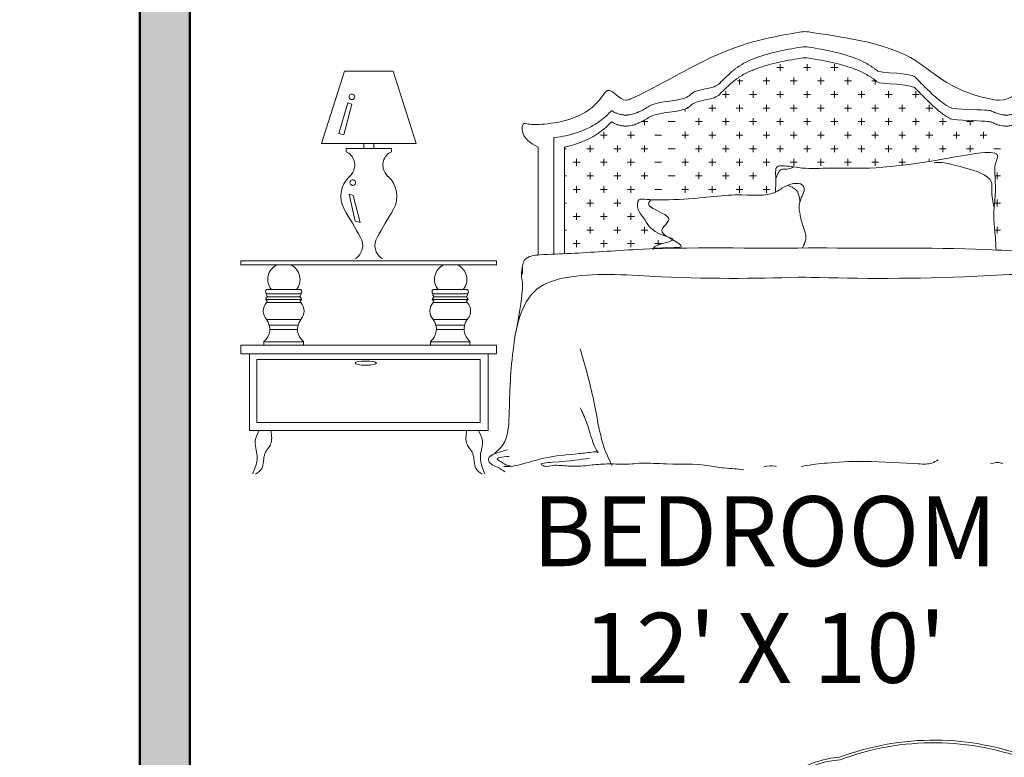
# Model space of a CAD drawing. Units: inches. Extents: x 1771 to 3025, y 319 to 889.
# Tile 33 of 35: x 2854 to 2952, y 714 to 788. Entities that reach past the tile are written whole.
import ezdxf

# ---------------------------------------------------------------- set-up
doc = ezdxf.new("R2010")
doc.units = ezdxf.units.IN
doc.header["$MEASUREMENT"] = 0
doc.set_wipeout_variables(frame=1)
for name, color, linetype, lineweight in [('A-AREA-IDEN', 241, 'Continuous', 25), ('A-FURN', 8, 'Continuous', 18), ('A-WALL', 7, 'Continuous', 50), ('A-WALL-PATT', 254, 'Continuous', 13)]:
    doc.layers.add(name, color=color, linetype=linetype, lineweight=lineweight)
doc.styles.get("Standard").update_dxf_attribs({"font": 'arial.ttf'})

# ---------------------------------------------------------------- blocks, each defined once
blk = doc.blocks.new('A$C3F6F0378')
for p, q in [((1198.7, 944.7), (1198.7, 946.2)), ((1254.2, 952.6), (1270.1, 952.6)), ((1262.2, 944.7), (1262.2, 960.5)), ((1317.7, 952.6), (1333.6, 952.6)), ((1325.7, 944.7), (1325.7, 960.5)), ((1381.2, 952.6), (1397.1, 952.6)), ((1389.2, 944.7), (1389.2, 959.9)), ((188.6, 774.2), (242.7, 943.6)), ((356.2, 943.6), (242.7, 943.6)), ((410.4, 774.2), (356.2, 943.6)), ((1166.9, 912.9), (1166.9, 924)), ((1230.4, 912.9), (1230.4, 928.8)), ((1293.9, 912.9), (1293.9, 928.8)), ((1357.4, 912.9), (1357.4, 928.8)), ((1420.9, 912.9), (1420.9, 928.8)), ((1162.7, 920.9), (1174.9, 920.9)), ((1222.5, 920.9), (1238.4, 920.9)), ((1286, 920.9), (1301.9, 920.9)), ((1349.5, 920.9), (1365.4, 920.9)), ((1413, 920.9), (1428.9, 920.9)), ((1476.5, 920.9), (1485.8, 920.9)), ((1484.4, 912.9), (1484.4, 921.6)), ((1127.2, 889.1), (1143.1, 889.1)), ((1135.2, 881.2), (1135.2, 897)), ((1190.7, 889.1), (1206.6, 889.1)), ((1198.7, 881.2), (1198.7, 897)), ((1254.2, 889.1), (1270.1, 889.1)), ((1262.2, 881.2), (1262.2, 897)), ((1317.7, 889.1), (1333.6, 889.1)), ((1325.7, 881.2), (1325.7, 897)), ((1381.2, 889.1), (1397.1, 889.1)), ((1389.2, 881.2), (1389.2, 897)), ((1444.7, 889.1), (1460.6, 889.1)), ((1452.7, 881.2), (1452.7, 897)), ((1508.2, 889.1), (1524.1, 889.1)), ((1516.2, 881.2), (1516.2, 897)), ((1571.7, 889.1), (1587.6, 889.1)), ((1579.7, 881.2), (1579.7, 897)), ((229, 797.8), (250.3, 869.3)), ((259.4, 866.2), (241.2, 794.8)), ((250.3, 869.3), (259.4, 866.2)), ((1039.9, 849.4), (1039.9, 855.2)), ((1044.6, 857.4), (1047.9, 857.4)), ((1095.5, 857.4), (1111.4, 857.4)), ((1103.4, 849.4), (1103.4, 865.3)), ((1159, 857.4), (1174.9, 857.4)), ((1166.9, 849.4), (1166.9, 865.3)), ((1222.5, 857.4), (1238.4, 857.4)), ((1230.4, 849.4), (1230.4, 865.3)), ((1286, 857.4), (1301.9, 857.4)), ((1293.9, 849.4), (1293.9, 865.3)), ((1349.5, 857.4), (1365.4, 857.4)), ((1357.4, 849.4), (1357.4, 865.3)), ((1413, 857.4), (1428.9, 857.4)), ((1420.9, 849.4), (1420.9, 865.3)), ((1476.5, 857.4), (1492.4, 857.4)), ((1484.4, 849.4), (1484.4, 865.3)), ((1540, 857.4), (1555.9, 857.4)), ((1547.9, 849.4), (1547.9, 865.3)), ((1603.5, 857.4), (1619.4, 857.4)), ((1611.4, 849.4), (1611.4, 865.3)), ((1071.7, 817.7), (1071.7, 833.5)), ((1135.2, 817.7), (1135.2, 833.5)), ((1198.7, 817.7), (1198.7, 833.5)), ((1262.2, 817.7), (1262.2, 833.5)), ((1325.7, 817.7), (1325.7, 833.5)), ((1389.2, 817.7), (1389.2, 833.5)), ((1452.7, 817.7), (1452.7, 833.5)), ((1516.2, 817.7), (1516.2, 833.5)), ((1579.7, 817.7), (1579.7, 833.5)), ((1643.2, 817.7), (1643.2, 833.5)), ((881.2, 817.7), (881.2, 818.8)), ((937.5, 825.6), (952.6, 825.6)), ((944.7, 817.7), (944.7, 829.4)), ((1000.2, 825.6), (1016.1, 825.6)), ((1063.7, 825.6), (1079.6, 825.6)), ((1127.2, 825.6), (1143.1, 825.6)), ((1190.7, 825.6), (1206.6, 825.6)), ((1254.2, 825.6), (1270.1, 825.6)), ((1317.7, 825.6), (1333.6, 825.6)), ((1381.2, 825.6), (1397.1, 825.6)), ((1444.7, 825.6), (1460.6, 825.6)), ((1508.2, 825.6), (1524.1, 825.6)), ((1571.7, 825.6), (1587.6, 825.6)), ((1635.2, 825.6), (1651.1, 825.6)), ((1698.7, 825.6), (1714.6, 825.6)), ((1706.7, 817.7), (1706.7, 828.2)), ((1770.2, 818.9), (1770.2, 818.9)), ((241.2, 794.8), (229, 797.8)), ((841.5, 793.9), (857.4, 793.9)), ((849.4, 785.9), (849.4, 801.8)), ((905, 793.9), (920.9, 793.9)), ((912.9, 785.9), (912.9, 801.8)), ((968.5, 793.9), (984.4, 793.9)), ((1032, 793.9), (1047.9, 793.9)), ((1039.9, 785.9), (1039.9, 801.8)), ((1095.5, 793.9), (1111.4, 793.9)), ((1103.4, 785.9), (1103.4, 801.8)), ((1159, 793.9), (1174.9, 793.9)), ((1166.9, 785.9), (1166.9, 801.8)), ((1222.5, 793.9), (1238.4, 793.9)), ((1230.4, 785.9), (1230.4, 801.8)), ((1286, 793.9), (1301.9, 793.9)), ((1293.9, 785.9), (1293.9, 801.8)), ((1349.5, 793.9), (1365.4, 793.9)), ((1357.4, 785.9), (1357.4, 801.8)), ((1413, 793.9), (1428.9, 793.9)), ((1420.9, 785.9), (1420.9, 801.8)), ((1476.5, 793.9), (1492.4, 793.9)), ((1484.4, 785.9), (1484.4, 801.8)), ((1540, 793.9), (1555.9, 793.9)), ((1547.9, 785.9), (1547.9, 801.8)), ((1603.5, 793.9), (1619.4, 793.9)), ((1611.4, 785.9), (1611.4, 801.8)), ((1667, 793.9), (1682.9, 793.9)), ((1674.9, 785.9), (1674.9, 801.8)), ((1730.5, 793.9), (1746.4, 793.9)), ((1738.4, 785.9), (1738.4, 801.8)), ((410.4, 774.2), (188.6, 774.2)), ((246.2, 763), (246.2, 755.2)), ((246.2, 763), (246.2, 755.2)), ((352.5, 763), (246.2, 763)), ((287.7, 774.2), (287.7, 763)), ((311, 763), (287.7, 763)), ((311, 774.2), (311, 763)), ((352.5, 763), (352.5, 755.2)), ((352.5, 763), (352.5, 755.2)), ((757.1, 762.1), (762.1, 762.1)), ((809.7, 762.1), (825.6, 762.1)), ((817.7, 754.2), (817.7, 770)), ((873.2, 762.1), (889.1, 762.1)), ((881.2, 754.2), (881.2, 770)), ((936.7, 762.1), (952.6, 762.1)), ((944.7, 754.2), (944.7, 770)), ((1000.2, 762.1), (1016.1, 762.1)), ((1063.7, 762.1), (1079.6, 762.1)), ((1071.7, 754.2), (1071.7, 770)), ((1127.2, 762.1), (1143.1, 762.1)), ((1135.2, 754.2), (1135.2, 770)), ((1190.7, 762.1), (1206.6, 762.1)), ((1198.7, 754.2), (1198.7, 770)), ((1254.2, 762.1), (1270.1, 762.1)), ((1262.2, 754.2), (1262.2, 770)), ((1317.7, 762.1), (1333.6, 762.1)), ((1325.7, 754.2), (1325.7, 770)), ((1381.2, 762.1), (1397.1, 762.1)), ((1389.2, 754.2), (1389.2, 770)), ((1444.7, 762.1), (1460.6, 762.1)), ((1452.7, 754.2), (1452.7, 770)), ((1508.2, 762.1), (1524.1, 762.1)), ((1516.2, 754.2), (1516.2, 770)), ((1571.7, 762.1), (1587.6, 762.1)), ((1579.7, 754.2), (1579.7, 770)), ((1635.2, 762.1), (1651.1, 762.1)), ((1643.2, 754.2), (1643.2, 770)), ((1698.7, 762.1), (1714.6, 762.1)), ((1706.7, 754.2), (1706.7, 770)), ((1762.2, 762.1), (1778.1, 762.1)), ((785.9, 722.4), (785.9, 738.3)), ((849.4, 722.4), (849.4, 738.3)), ((912.9, 722.4), (912.9, 738.3)), ((1039.9, 722.4), (1039.9, 738.3)), ((1103.4, 722.4), (1103.4, 738.3)), ((1166.9, 722.4), (1166.9, 738.3)), ((1230.4, 722.4), (1230.4, 738.3)), ((1293.9, 722.4), (1293.9, 738.3)), ((1357.4, 722.4), (1357.4, 738.3)), ((1420.9, 722.4), (1420.9, 738.3)), ((1484.4, 722.4), (1484.4, 738.3)), ((1547.9, 723.4), (1547.9, 738.3)), ((1611.4, 732.6), (1611.4, 738.3)), ((778, 730.4), (793.9, 730.4)), ((841.5, 730.4), (857.4, 730.4)), ((905, 730.4), (920.9, 730.4)), ((968.5, 730.4), (984.4, 730.4)), ((1032, 730.4), (1047.9, 730.4)), ((1095.5, 730.4), (1111.4, 730.4)), ((1159, 730.4), (1174.9, 730.4)), ((1222.5, 730.4), (1238.4, 730.4)), ((1286, 730.4), (1301.9, 730.4)), ((1349.5, 730.4), (1365.4, 730.4)), ((1413, 730.4), (1428.9, 730.4)), ((1476.5, 730.4), (1492.4, 730.4)), ((1540, 730.4), (1555.9, 730.4)), ((757.1, 698.6), (762.1, 698.6)), ((809.7, 698.6), (825.6, 698.6)), ((817.7, 690.7), (817.7, 706.5)), ((873.2, 698.6), (889.1, 698.6)), ((881.2, 690.7), (881.2, 706.5)), ((936.7, 698.6), (952.6, 698.6)), ((944.7, 690.7), (944.7, 706.5)), ((1000.2, 698.6), (1016.1, 698.6)), ((1063.7, 698.6), (1079.6, 698.6)), ((1071.7, 690.7), (1071.7, 706.5)), ((1127.2, 698.6), (1143.1, 698.6)), ((1135.2, 690.7), (1135.2, 706.5)), ((1190.7, 698.6), (1206.6, 698.6)), ((1198.7, 690.7), (1198.7, 706.5)), ((1765.2, 698.6), (1778.1, 698.6)), ((1770.2, 690.7), (1770.2, 706.5)), ((785.9, 658.9), (785.9, 674.8)), ((849.4, 658.9), (849.4, 674.8)), ((912.9, 658.9), (912.9, 674.8)), ((1039.9, 658.9), (1039.9, 674.8)), ((1103.4, 658.9), (1103.4, 674.8)), ((1166.9, 658.9), (1166.9, 674.8)), ((1230.4, 658.9), (1230.4, 674.8)), ((253.5, 655.6), (262.6, 652.5)), ((267.2, 592.3), (253.5, 655.6)), ((262.6, 652.5), (279.4, 589.2)), ((778, 666.9), (793.9, 666.9)), ((841.5, 666.9), (857.4, 666.9)), ((905, 666.9), (920.9, 666.9)), ((968.5, 666.9), (984.4, 666.9)), ((1032, 666.9), (1047.9, 666.9)), ((1095.5, 666.9), (1111.4, 666.9)), ((1159, 666.9), (1174.9, 666.9)), ((1222.5, 666.9), (1238.4, 666.9)), ((757.1, 635.1), (762.1, 635.1)), ((809.7, 635.1), (825.6, 635.1)), ((817.7, 627.2), (817.7, 643)), ((873.2, 635.1), (889.1, 635.1)), ((881.2, 627.2), (881.2, 643)), ((1764.2, 635.1), (1778.1, 635.1)), ((1770.2, 627.2), (1770.2, 643)), ((778, 603.4), (793.9, 603.4)), ((785.9, 595.4), (785.9, 611.3)), ((841.5, 603.4), (857.4, 603.4)), ((849.4, 595.4), (849.4, 611.3)), ((905, 603.4), (920.9, 603.4)), ((912.9, 595.4), (912.9, 611.3)), ((279.4, 589.2), (267.2, 592.3)), ((817.7, 563.7), (817.7, 579.5)), ((881.2, 563.7), (881.2, 579.5)), ((944.7, 563.7), (944.7, 579.5)), ((1770.2, 563.7), (1770.2, 579.5)), ((757.1, 571.6), (762.1, 571.6)), ((809.7, 571.6), (825.6, 571.6)), ((873.2, 571.6), (889.1, 571.6)), ((936.7, 571.6), (952.6, 571.6)), ((1764.5, 571.6), (1778.1, 571.6)), ((778, 539.9), (793.9, 539.9)), ((785.9, 531.9), (785.9, 547.8)), ((841.5, 539.9), (857.4, 539.9)), ((849.4, 531.9), (849.4, 547.8)), ((905, 539.9), (920.9, 539.9)), ((912.9, 531.9), (912.9, 547.8)), ((968.5, 539.9), (984.4, 539.9)), ((976.4, 536.8), (976.4, 547.8)), ((598.4, 500), (0, 500)), ((0, 499.7), (0, 489.7)), ((598.4, 490), (0, 490)), ((598.4, 499.7), (598.4, 489.7)), ((658.9, 468.4), (658.9, 484.3)), ((140, 432.2), (60, 432.2)), ((140, 432.2), (60, 432.2)), ((140, 422.2), (60, 422.2)), ((138.2, 415.4), (61.8, 415.4)), ((529.9, 432.2), (449.9, 432.2)), ((529.9, 432.2), (449.9, 432.2)), ((529.9, 422.2), (449.9, 422.2)), ((528.1, 415.4), (451.7, 415.4)), ((141.9, 409.3), (58.1, 409.3)), ((140, 402.2), (60, 402.2)), ((531.8, 409.3), (447.9, 409.3)), ((529.9, 402.2), (449.9, 402.2)), ((140, 362.2), (60, 362.2)), ((133.7, 349.2), (66.3, 349.2)), ((529.9, 362.2), (449.9, 362.2)), ((523.5, 349.2), (456.2, 349.2)), ((132.4, 338.7), (67.5, 338.7)), ((522.3, 338.7), (457.4, 338.7)), ((0, 302.2), (0, 282.2)), ((598.4, 302.2), (0, 302.2)), ((53.7, 311), (53.7, 302.2)), ((146.3, 310.3), (53.7, 310.3)), ((80, 302.2), (120, 302.2)), ((80, 302.2), (130, 302.2)), ((146.3, 311), (146.3, 302.2)), ((443.6, 311), (443.6, 302.2)), ((536.1, 310.3), (443.6, 310.3)), ((469.9, 302.2), (509.9, 302.2)), ((469.9, 302.2), (519.9, 302.2)), ((536.1, 311), (536.1, 302.2)), ((598.4, 282.2), (598.4, 302.2)), ((598.4, 282.2), (0, 282.2)), ((20, 282.2), (20, 102.2)), ((578.4, 102.2), (578.4, 282.2)), ((37.2, 268.9), (560.2, 268.9)), ((37.2, 120.8), (37.2, 268.9)), ((560.2, 268.9), (560.2, 120.8)), ((560.2, 120.8), (37.2, 120.8)), ((20, 102.2), (578.4, 102.2))]:
    blk.add_line(p, q)
at = {"ltscale": 20}
for p, q in [((732.5, 788.3), (732.5, 515.5)), ((695.7, 766.2), (695.7, 513.2)), ((757.1, 766), (757.1, 516.6))]:
    blk.add_line(p, q, dxfattribs=at)
for centre in [(1320.3, 981.3), (1320.4, 945.7), (1320.4, 919.9)]:
    blk.add_arc(centre, 55.2, 80.5605, 99.4395, dxfattribs=at)
for centre, radius, start, end in [((259.7, 883.6), 6.48, 168.6084, 233.2112), ((259.7, 883.6), 6.49, 104.0344, 168.6084), ((259.6, 883.5), 6.42, 233.2112, 255.9722), ((260, 883.6), 6.51, 78.6968, 107.1924), ((259.7, 883.8), 6.69, 255.9722, 278.2688), ((259.7, 883.9), 6.81, 278.2688, 342.9026), ((260, 883.7), 6.5, 50.1648, 78.6968), ((260.1, 883.8), 6.35, 342.9026, 50.1648), ((232.6, 724.1), 33.9, 326.6744, 66.3416), ((366.1, 724.1), 33.9, 113.6584, 213.3256), ((295.2, 651.2), 61.5, 132.0366, 209.8723), ((231, 722.3), 34.4, 312.0366, 330.6067), ((367.7, 722.3), 34.4, 209.3933, 227.9634), ((303.6, 651.2), 61.5, 330.1277, 47.9634), ((261.7, 682.8), 6.48, 168.6084, 233.2112), ((261.7, 682.8), 6.49, 104.0344, 168.6084), ((261.6, 682.8), 6.42, 233.2112, 255.9722), ((262, 682.9), 6.51, 78.6968, 107.1924), ((261.7, 683), 6.69, 255.9722, 278.2688), ((261.7, 683.1), 6.81, 278.2688, 342.9026), ((262, 682.9), 6.5, 50.1648, 78.6968), ((262.1, 683), 6.35, 342.9026, 50.1648), ((9112.8, 5715.8), 10230.1, 209.87228, 210.29853), ((-8514, 5715.8), 10230.1, 329.70147, 330.12772), ((247.8, 535.9), 37.3, 302.5427, 30.2985), ((350.9, 535.9), 37.3, 149.7015, 237.4573), ((100.5, 456.1), 37.8, 115.9414, 219.2084), ((100.5, 456.1), 37.8, 320.7916, 64.0586), ((490.9, 456.1), 37.8, 115.9414, 219.2084), ((490.9, 456.1), 37.8, 320.7916, 64.0586), ((63.7, 427.2), 6.24, 126.78, 233.22), ((136.2, 427.2), 6.24, 306.78, 53.22), ((453.6, 427.2), 6.24, 126.78, 233.22), ((526.1, 427.2), 6.24, 306.78, 53.22), ((82, 382.2), 29.7, 137.7452, 222.2548), ((118, 382.2), 29.7, 317.7452, 42.2548), ((471.9, 382.2), 29.7, 137.7452, 222.2548), ((507.8, 382.2), 29.7, 317.7452, 42.2548), ((30.6, 339.8), 37, 308.7547, 37.2668), ((169.4, 339.8), 37, 142.7332, 231.2453), ((420.5, 339.8), 37, 308.7547, 37.2668), ((559.3, 339.8), 37, 142.7332, 231.2453)]:
    blk.add_arc(centre, radius, start, end)
blk.add_ellipse((292.3, 260.1), major_axis=(25, 0), ratio=0.2)
for points, knots in [([(695.7, 766.2), (675.2, 775.8), (657.2, 791.6), (658.6, 824.3), (675.7, 817.9), (731.9, 819.9), (817.7, 836.7), (863.4, 913.8), (889.3, 869.9), (957.4, 896.6), (1128.9, 1003.6), (1245.7, 1025), (1311.4, 1035.8)], [12.417853, 12.417853, 12.417853, 12.417853, 68.394536, 90.665986, 114.156853, 157.554067, 281.869614, 298.858744, 338.737111, 347.060176, 470.423438, 625.498764, 625.498764, 625.498764, 625.498764]), ([(1996.6, 766.2), (2017.1, 775.8), (2035.1, 791.6), (2033.8, 824.3), (2016.6, 817.9), (1960.4, 819.9), (1874.7, 836.7), (1829, 913.8), (1803, 869.9), (1652.5, 896.6), (1584, 1003.6), (1395.1, 1025), (1329.4, 1035.8)], [12.417853, 12.417853, 12.417853, 12.417853, 68.394536, 90.665986, 114.156853, 157.554067, 281.869614, 298.858744, 338.737111, 347.060176, 470.423438, 625.498764, 625.498764, 625.498764, 625.498764]), ([(867.4, 851.3), (868.1, 850.9), (868.9, 850.4), (871.2, 849.1), (872.9, 848.2), (876.8, 846.3), (879, 845.4), (884, 843.6), (886.7, 842.8), (892, 841.7), (894.6, 841.4), (898.4, 841.1), (899.4, 841), (901.2, 841), (901.9, 841), (903.1, 841), (903.7, 841.1), (904.8, 841.1), (905.4, 841.2), (907, 841.3), (908.1, 841.4), (911.6, 841.9), (913.8, 842.3), (917.8, 843.3), (919.6, 843.9), (922.7, 844.9), (924.1, 845.5), (926.6, 846.4), (927.6, 846.9), (928.8, 847.4), (929.1, 847.5), (929.7, 847.8), (929.9, 847.9), (930.7, 848.2), (931.3, 848.5), (932.9, 849.2), (933.9, 849.7), (937.1, 851.3), (939.2, 852.3), (945.3, 855.5), (949.2, 857.8), (959.8, 864.4), (966.2, 869), (1040, 878.3), (1045.6, 883.1), (1056.3, 892.7), (1061.3, 897.5), (1112.2, 907), (1116.8, 911.6), (1125.6, 920.6), (1129.9, 924.9), (1138.3, 933), (1142.3, 936.8), (1148.2, 942), (1150, 943.5), (1153.3, 946.3), (1154.7, 947.4), (1157, 949.2), (1157.9, 949.9), (1159.7, 951.2), (1160.6, 951.8), (1163.4, 953.8), (1165.3, 955), (1171, 958.7), (1174.9, 961), (1186, 967), (1193.5, 970.4), (1209.3, 976.7), (1217.6, 979.5), (1235, 984.7), (1244, 987), (1262.7, 991.3), (1272.4, 993.3), (1291.8, 996.9), (1301.5, 998.6), (1311.3, 1000.2)], [328.6705, 328.6705, 328.6705, 328.6705, 329.609368, 329.609368, 331.487103, 331.487103, 333.620342, 333.620342, 335.753581, 335.753581, 337.507866, 337.507866, 338.182373, 338.182373, 338.607397, 338.607397, 338.959312, 338.959312, 339.311227, 339.311227, 340.015058, 340.015058, 341.722742, 341.722742, 343.430427, 343.430427, 345.138111, 345.138111, 346.845796, 346.845796, 347.37881, 347.37881, 347.911824, 347.911824, 348.977853, 348.977853, 351.109909, 351.109909, 355.374023, 355.374023, 363.902249, 363.902249, 379.258481, 379.258481, 394.614712, 394.614712, 409.970944, 409.970944, 425.327175, 425.327175, 440.683406, 440.683406, 456.039638, 456.039638, 463.285514, 463.285514, 469.01116, 469.01116, 472.593, 472.593, 476.17484, 476.17484, 483.338521, 483.338521, 497.665882, 497.665882, 522.309302, 522.309302, 546.952723, 546.952723, 571.596143, 571.596143, 596.239564, 596.239564, 619.876409, 619.876409, 619.876409, 619.876409]), ([(1824.9, 851.3), (1824.2, 850.9), (1823.5, 850.4), (1821.1, 849.1), (1819.5, 848.2), (1815.6, 846.3), (1813.3, 845.4), (1808.4, 843.6), (1805.7, 842.8), (1800.3, 841.7), (1797.7, 841.4), (1794, 841.1), (1792.9, 841), (1791.2, 841), (1790.5, 841), (1789.2, 841), (1788.6, 841.1), (1787.5, 841.1), (1787, 841.2), (1785.3, 841.3), (1784.3, 841.4), (1780.8, 841.9), (1778.6, 842.3), (1774.6, 843.3), (1772.8, 843.9), (1769.6, 844.9), (1768.2, 845.5), (1765.8, 846.4), (1764.7, 846.9), (1763.5, 847.4), (1763.2, 847.5), (1762.7, 847.8), (1762.4, 847.9), (1761.6, 848.2), (1761.1, 848.5), (1759.5, 849.2), (1758.4, 849.7), (1755.2, 851.3), (1753.2, 852.3), (1664.6, 855.5), (1660.7, 857.8), (1650.1, 864.4), (1643.7, 869), (1631.7, 878.3), (1626.1, 883.1), (1615.5, 892.7), (1610.4, 897.5), (1600.8, 907), (1596.2, 911.6), (1587.3, 920.6), (1583, 924.9), (1574.7, 933), (1570.6, 936.8), (1492.6, 942), (1490.8, 943.5), (1487.5, 946.3), (1486.1, 947.4), (1483.8, 949.2), (1482.9, 949.9), (1481.1, 951.2), (1480.2, 951.8), (1477.4, 953.8), (1475.5, 955), (1469.8, 958.7), (1465.9, 961), (1454.8, 967), (1447.3, 970.4), (1431.5, 976.7), (1423.2, 979.5), (1405.8, 984.7), (1396.8, 987), (1378.1, 991.3), (1368.4, 993.3), (1349, 996.9), (1339.3, 998.6), (1329.5, 1000.2)], [328.6705, 328.6705, 328.6705, 328.6705, 329.609368, 329.609368, 331.487103, 331.487103, 333.620342, 333.620342, 335.753581, 335.753581, 337.507866, 337.507866, 338.182373, 338.182373, 338.607397, 338.607397, 338.959312, 338.959312, 339.311227, 339.311227, 340.015058, 340.015058, 341.722742, 341.722742, 343.430427, 343.430427, 345.138111, 345.138111, 346.845796, 346.845796, 347.37881, 347.37881, 347.911824, 347.911824, 348.977853, 348.977853, 351.109909, 351.109909, 355.374023, 355.374023, 363.902249, 363.902249, 379.258481, 379.258481, 394.614712, 394.614712, 409.970943, 409.970943, 425.327175, 425.327175, 440.683406, 440.683406, 456.039637, 456.039637, 463.285514, 463.285514, 469.011154, 469.011154, 472.592992, 472.592992, 476.17483, 476.17483, 483.338506, 483.338506, 497.665857, 497.665857, 522.309275, 522.309275, 546.952693, 546.952693, 571.59611, 571.59611, 596.239528, 596.239528, 619.876409, 619.876409, 619.876409, 619.876409]), ([(867.4, 825.4), (868.1, 825), (868.9, 824.6), (871.2, 823.2), (872.9, 822.3), (876.8, 820.5), (879, 819.5), (884, 817.8), (886.7, 817), (892, 815.9), (894.6, 815.5), (898.4, 815.2), (899.4, 815.2), (901.2, 815.2), (901.9, 815.2), (903.1, 815.2), (903.7, 815.2), (904.8, 815.3), (905.4, 815.3), (907, 815.4), (908.1, 815.5), (911.6, 816), (913.8, 816.5), (917.8, 817.5), (919.6, 818), (922.7, 819.1), (924.1, 819.6), (926.6, 820.6), (927.6, 821), (928.8, 821.5), (929.1, 821.7), (929.7, 821.9), (929.9, 822), (930.7, 822.4), (931.3, 822.6), (932.9, 823.4), (933.9, 823.9), (937.1, 825.4), (939.2, 826.4), (945.3, 829.7), (949.2, 832), (959.8, 838.6), (966.2, 843.1), (1040, 852.4), (1045.6, 857.2), (1056.3, 866.8), (1061.3, 871.6), (1112.2, 881.1), (1116.8, 885.7), (1125.6, 894.7), (1129.9, 899), (1138.3, 907.1), (1142.3, 910.9), (1148.2, 916.1), (1150, 917.7), (1153.3, 920.4), (1154.7, 921.5), (1157, 923.3), (1157.9, 924), (1159.7, 925.3), (1160.6, 926), (1163.4, 927.9), (1165.3, 929.2), (1171, 932.8), (1174.9, 935.2), (1186, 941.1), (1193.5, 944.6), (1209.3, 950.8), (1217.6, 953.7), (1235, 958.8), (1244, 961.2), (1262.7, 965.5), (1272.4, 967.4), (1291.8, 971), (1301.5, 972.7), (1311.3, 974.3)], [328.6705, 328.6705, 328.6705, 328.6705, 329.609368, 329.609368, 331.487103, 331.487103, 333.620342, 333.620342, 335.753581, 335.753581, 337.507866, 337.507866, 338.182373, 338.182373, 338.607397, 338.607397, 338.959312, 338.959312, 339.311227, 339.311227, 340.015058, 340.015058, 341.722742, 341.722742, 343.430427, 343.430427, 345.138111, 345.138111, 346.845796, 346.845796, 347.37881, 347.37881, 347.911824, 347.911824, 348.977853, 348.977853, 351.109909, 351.109909, 355.374023, 355.374023, 363.902249, 363.902249, 379.258481, 379.258481, 394.614712, 394.614712, 409.970944, 409.970944, 425.327175, 425.327175, 440.683406, 440.683406, 456.039638, 456.039638, 463.285514, 463.285514, 469.01116, 469.01116, 472.593, 472.593, 476.17484, 476.17484, 483.338521, 483.338521, 497.665882, 497.665882, 522.309302, 522.309302, 546.952723, 546.952723, 571.596143, 571.596143, 596.239564, 596.239564, 619.876409, 619.876409, 619.876409, 619.876409]), ([(1824.9, 825.4), (1824.2, 825), (1823.5, 824.6), (1821.1, 823.2), (1819.5, 822.3), (1815.6, 820.5), (1813.3, 819.5), (1808.4, 817.8), (1805.7, 817), (1800.3, 815.9), (1797.7, 815.5), (1794, 815.2), (1792.9, 815.2), (1791.2, 815.2), (1790.5, 815.2), (1789.2, 815.2), (1788.6, 815.2), (1787.5, 815.3), (1787, 815.3), (1785.3, 815.4), (1784.3, 815.5), (1780.8, 816), (1778.6, 816.5), (1774.6, 817.5), (1772.8, 818), (1769.6, 819.1), (1768.2, 819.6), (1765.8, 820.6), (1764.7, 821), (1763.5, 821.5), (1763.2, 821.7), (1762.7, 821.9), (1762.4, 822), (1761.6, 822.4), (1761.1, 822.6), (1759.5, 823.4), (1758.4, 823.9), (1755.2, 825.4), (1753.2, 826.4), (1664.6, 829.7), (1660.7, 832), (1650.1, 838.6), (1643.7, 843.1), (1631.7, 852.4), (1626.1, 857.2), (1615.5, 866.8), (1610.4, 871.6), (1600.8, 881.1), (1596.2, 885.7), (1587.3, 894.7), (1583, 899), (1574.7, 907.1), (1570.6, 910.9), (1492.6, 916.1), (1490.8, 917.7), (1487.5, 920.4), (1486.1, 921.5), (1483.8, 923.3), (1482.9, 924), (1481.1, 925.3), (1480.2, 926), (1477.4, 927.9), (1475.5, 929.2), (1469.8, 932.8), (1465.9, 935.2), (1454.8, 941.1), (1447.3, 944.6), (1431.5, 950.8), (1423.2, 953.7), (1405.8, 958.8), (1396.8, 961.2), (1378.1, 965.5), (1368.4, 967.4), (1349, 971), (1339.3, 972.7), (1329.5, 974.3)], [328.6705, 328.6705, 328.6705, 328.6705, 329.609368, 329.609368, 331.487103, 331.487103, 333.620342, 333.620342, 335.753581, 335.753581, 337.507866, 337.507866, 338.182373, 338.182373, 338.607397, 338.607397, 338.959312, 338.959312, 339.311227, 339.311227, 340.015058, 340.015058, 341.722742, 341.722742, 343.430427, 343.430427, 345.138111, 345.138111, 346.845796, 346.845796, 347.37881, 347.37881, 347.911824, 347.911824, 348.977853, 348.977853, 351.109909, 351.109909, 355.374023, 355.374023, 363.902249, 363.902249, 379.258481, 379.258481, 394.614712, 394.614712, 409.970943, 409.970943, 425.327175, 425.327175, 440.683406, 440.683406, 456.039637, 456.039637, 463.285514, 463.285514, 469.011154, 469.011154, 472.592992, 472.592992, 476.17483, 476.17483, 483.338506, 483.338506, 497.665857, 497.665857, 522.309275, 522.309275, 546.952693, 546.952693, 571.59611, 571.59611, 596.239528, 596.239528, 619.876409, 619.876409, 619.876409, 619.876409]), ([(732.5, 788.3), (744.7, 789.4), (752.5, 790.8), (768.6, 794.5), (777, 796.7), (793.9, 802.3), (802.4, 805.7), (819.3, 813.7), (827.7, 818.4), (842.6, 828.5), (849.2, 833.6), (859.6, 843.1), (863.6, 847.1), (867.4, 851.3)], [179.330708, 179.330708, 179.330708, 179.330708, 196.086144, 196.086144, 213.445516, 213.445516, 230.804888, 230.804888, 248.16426, 248.16426, 262.451931, 262.451931, 271.832526, 271.832526, 271.832526, 271.832526]), ([(757.1, 766), (758.2, 766.3), (759.3, 766.5), (768.6, 768.6), (777, 770.9), (793.9, 776.5), (802.4, 779.8), (819.3, 787.9), (827.7, 792.6), (842.6, 802.7), (849.2, 807.8), (859.6, 817.2), (863.6, 821.2), (867.4, 825.4)], [193.740688, 193.740688, 193.740688, 193.740688, 196.086144, 196.086144, 213.445516, 213.445516, 230.804888, 230.804888, 248.16426, 248.16426, 262.451931, 262.451931, 271.832526, 271.832526, 271.832526, 271.832526])]:
    blk.add_open_spline(points, degree=3, knots=knots, dxfattribs=at)
at = {"ltscale": 5}
for points, knots in [([(1251.5, 660.5), (1251.8, 673.8), (1252.2, 692.2), (1250.9, 722.8), (1282.7, 722.3), (1319.1, 713.9), (1424.2, 721.3), (1489.1, 705.6), (1786.5, 765.5), (1764.9, 728.8), (1764.7, 698.2), (1767.9, 658.9), (1761, 614.3), (1764.1, 574.4), (1766.6, 548.7), (1767.9, 525.2)], [3.603347, 3.603347, 3.603347, 3.603347, 60.838375, 82.182907, 107.012175, 163.177093, 249.239778, 501.114283, 577.787612, 607.274607, 630.949286, 706.159707, 762.92633, 812.910096, 867.096105, 867.096105, 867.096105, 867.096105]), ([(1293.1, 719.7), (1288.2, 716.8), (1279.1, 713), (1263.5, 715.9), (1256.5, 703.2), (1253.3, 695), (1251.9, 690.7)], [16.588235, 16.588235, 16.588235, 16.588235, 39.368234, 56.465167, 72.647278, 91.317886, 91.317886, 91.317886, 91.317886]), ([(1623.4, 730.2), (1631.2, 730.2), (1644.4, 730.3), (1665.2, 725.1), (1763.6, 700.2), (1754.4, 664.8), (1760.1, 637.6), (1763, 624), (1763.1, 623.6)], [0, 0, 0, 0, 31.268494, 53.71641, 83.24833, 138.583941, 192.96698, 194.695488, 194.695488, 194.695488, 194.695488]), ([(964.3, 525.7), (965, 536.9), (1030.6, 547.7), (956.6, 565.4), (948, 599.2), (929.2, 612.7), (925.7, 647.1), (951.8, 642.5), (1054.9, 642.1), (1162.4, 661.2), (1239, 646.9), (1276.3, 678.9), (1316.3, 686.5), (1319.5, 660.6), (1309.9, 647.1), (1305, 623.9), (1309.2, 608.7), (1312.5, 586.6), (1326.7, 553.1), (1318.1, 538.8), (1314.8, 529.7)], [33.020195, 33.020195, 33.020195, 33.020195, 57.294753, 90.473933, 194.149416, 257.058105, 304.592565, 338.383824, 389.043604, 577.649845, 759.359611, 813.032269, 898.973184, 920.659088, 956.429806, 1000.911745, 1042.797508, 1121.842246, 1191.460876, 1213.109701, 1213.109701, 1213.109701, 1213.109701]), ([(1278.5, 676.1), (1286.8, 673.9), (1304.1, 667.4), (1307.6, 649.1), (1308.3, 637.8)], [13.535772, 13.535772, 13.535772, 13.535772, 45.871957, 87.312392, 87.312392, 87.312392, 87.312392]), ([(961.3, 642.9), (955.5, 638.3), (944, 626.2), (1030.7, 599.4), (953, 567.4), (1038.4, 539.7), (1029.3, 530.5), (966, 529.3)], [5.952535, 5.952535, 5.952535, 5.952535, 29.258845, 70.114919, 115.518645, 162.322231, 169.813565, 169.813565, 169.813565, 169.813565]), ([(643.4, 331.9), (665.9, 445.8), (654.5, 454.3), (658, 480.9), (661.2, 509.9), (714.1, 515.4), (786.5, 516.7), (1040.5, 536.6), (1224.6, 526.5), (1352.9, 530.4)], [0, 0, 0, 0, 32.681627, 48.455722, 75.25348, 112.004017, 183.381957, 310.642358, 688.088714, 688.088714, 688.088714, 688.088714]), ([(2022.3, 380), (2023.2, 448.3), (2041.3, 454.3), (2037.8, 480.9), (2034.7, 509.9), (1981.7, 515.4), (1909.3, 516.7), (1667.8, 533.2), (1476.1, 527.9), (1347.4, 530.2)], [0, 0, 0, 0, 32.681627, 48.455722, 75.25348, 112.004017, 183.381957, 310.642358, 588.939547, 588.939547, 588.939547, 588.939547]), ([(594.1, 49), (601.1, 55.3), (626, 78.1), (628.7, 172), (631.8, 287.1), (663.1, 436.6), (808.3, 475), (1037.5, 455.3), (1227.9, 458.5), (1322.1, 461.7)], [0, 0, 0, 0, 28.320233, 100.953775, 269.820348, 420.691469, 489.161544, 656.134073, 940.569207, 940.569207, 940.569207, 940.569207]), ([(2101.8, 49), (2094.8, 55.3), (2069.8, 78.1), (2053.9, 172), (2031.7, 287.1), (2023.3, 445.1), (1887.5, 475), (1637.7, 455.3), (1416.4, 458.5), (1314.5, 461.4)], [0, 0, 0, 0, 28.320233, 100.953775, 269.820348, 420.691469, 489.161544, 656.134073, 940.569207, 940.569207, 940.569207, 940.569207]), ([(794.2, 293.6), (806.6, 250.4), (830.4, 167.7), (842.1, 71.7), (865.2, 27.8), (869.1, 20.4)], [0, 0, 0, 0, 135.247847, 258.692787, 283.800228, 283.800228, 283.800228, 283.800228]), ([(794.2, 155.1), (799.6, 144.1), (814.7, 112.8), (821.4, 74.6), (834.4, 53), (835.9, 50.7)], [0, 0, 0, 0, 37.234018, 105.386078, 113.844905, 113.844905, 113.844905, 113.844905]), ([(624.2, 57.4), (618.3, 55.8), (603.1, 51.8), (572.2, 40.6), (586.5, 21.1), (602, 16.6), (612.3, 9.7), (617.8, 5.9)], [0, 0, 0, 0, 19.937155, 51.57724, 63.193909, 80.21631, 100.09061, 100.09061, 100.09061, 100.09061]), ([(615.5, 18.4), (620.3, 18.3), (633.7, 17.9), (664.9, 24.9), (717, 41.9), (776.4, 46.5), (816.6, 50.9), (832.8, 53.1), (835.5, 51), (835.9, 50.7)], [0, 0, 0, 0, 14.447875, 40.468341, 96.220884, 181.018327, 216.046098, 224.609189, 226.185962, 226.185962, 226.185962, 226.185962]), ([(628, 41.8), (612, 40.1), (592.4, 38.1), (608.5, 29.7), (617.4, 21.9), (627.8, 19.8), (634.3, 18.4)], [0, 0, 0, 0, 28.05485, 34.289435, 45.980108, 65.027556, 65.027556, 65.027556, 65.027556]), ([(815.7, 37.2), (795, 34.1), (767.8, 30.1), (693.6, 25.5), (716, 16.2), (729.8, 21.8), (754.8, 20), (787, 17), (826.3, 22.8), (869.3, 25.1), (905.1, 21.9), (935.5, 27.3), (1029.7, 21.6), (1063.4, 26), (1134.3, 13.3), (1155.4, 13.6), (1169.6, 10.9), (1177, 9.9)], [0, 0, 0, 0, 87.513803, 114.592793, 124.77702, 141.903576, 160.817021, 198.691115, 240.471478, 280.23486, 329.410006, 348.41762, 373.077233, 428.05708, 447.802257, 468.691939, 491.310217, 491.310217, 491.310217, 491.310217]), ([(1311.8, 17.5), (1313.3, 17.9), (1334, 23.1), (1377.5, 26.3), (1445.4, 32.7), (1573.8, 24.6), (1614, 23), (1627.1, 30.7), (1632, 33.6)], [590.079786, 590.079786, 590.079786, 590.079786, 594.646549, 651.888327, 725.747367, 797.841373, 826.274406, 843.189267, 843.189267, 843.189267, 843.189267]), ([(1754.5, 25.1), (1763.4, 26.5), (1773.5, 29), (1782.6, 25.5), (1783.6, 25.1)], [516.212662, 516.212662, 516.212662, 516.212662, 542.681017, 546.007116, 546.007116, 546.007116, 546.007116]), ([(1224.5, 17.5), (1233.4, 18.9), (1243.5, 21.4), (1252.6, 17.9), (1253.7, 17.5)], [516.212662, 516.212662, 516.212662, 516.212662, 542.681017, 546.007116, 546.007116, 546.007116, 546.007116])]:
    blk.add_open_spline(points, degree=3, knots=knots, dxfattribs=at)
for points, knots in [([(60, 422.2), (59.5, 421), (58.6, 418.8), (63.4, 417.1), (60.1, 412.9), (56.2, 408.7), (63.1, 405.7), (60.8, 403.1), (60, 402.2)], [0, 0, 0, 0, 3.125, 6.207289, 10.622222, 14.901958, 20.470919, 23.596268, 23.596268, 23.596268, 23.596268]), ([(140, 422.2), (140.5, 421), (141.4, 418.8), (136.6, 417.1), (139.8, 412.9), (143.7, 408.7), (136.9, 405.7), (139.2, 403.1), (140, 402.2)], [0, 0, 0, 0, 3.125, 6.207289, 10.622222, 14.901958, 20.470919, 23.596268, 23.596268, 23.596268, 23.596268]), ([(449.9, 422.2), (449.4, 421), (448.5, 418.8), (453.2, 417.1), (450, 412.9), (446.1, 408.7), (453, 405.7), (450.7, 403.1), (449.9, 402.2)], [0, 0, 0, 0, 3.125, 6.207289, 10.622222, 14.901958, 20.470919, 23.596268, 23.596268, 23.596268, 23.596268]), ([(529.8, 422.2), (530.3, 421), (531.3, 418.8), (526.5, 417.1), (529.7, 412.9), (533.6, 408.7), (526.8, 405.7), (529, 403.1), (529.8, 402.2)], [0, 0, 0, 0, 3.125, 6.207289, 10.622222, 14.901958, 20.470919, 23.596268, 23.596268, 23.596268, 23.596268]), ([(42.9, 101.6), (38.6, 94.2), (28.1, 75.7), (43.8, 40.1), (33.3, 14.7), (27.7, 0.9)], [0, 0, 0, 0, 24.696996, 61.099524, 104.177437, 104.177437, 104.177437, 104.177437]), ([(70.4, 101.6), (71.9, 90.6), (74.7, 70.5), (49.8, 47.4), (55.7, 15.4), (39.9, 4), (34.3, 0)], [0, 0, 0, 0, 31.35672, 56.935761, 92.890491, 112.386558, 112.386558, 112.386558, 112.386558]), ([(528.3, 101.6), (526.8, 90.6), (524.1, 70.5), (549, 47.4), (543, 15.4), (558.9, 4), (564.5, 0)], [0, 0, 0, 0, 31.35672, 56.935761, 92.890491, 112.386558, 112.386558, 112.386558, 112.386558]), ([(555.9, 101.6), (560.2, 94.2), (570.6, 75.7), (554.9, 40.1), (565.4, 14.7), (571.1, 0.9)], [0, 0, 0, 0, 24.696996, 61.099524, 104.177437, 104.177437, 104.177437, 104.177437])]:
    blk.add_open_spline(points, degree=3, knots=knots)
blk = doc.blocks.new('A$C425441F1')
for points in [[(1639.3, 0), (1667.3, 0), (1667.3, 55.3), (1748.6, 55.3), (1748.6, 807.4), (1761.1, 860.7), (1735.7, 880.7), (1703.4, 883.3), (1675.8, 879.6), (1656.2, 873.5), (1635.2, 863.3), (1619.6, 852.6), (1605.1, 839.5), (1596.7, 829.9), (1583.2, 810), (1573.2, 788.1), (1567.6, 767.7), (1566.5, 761.6), (1541.6, 750.9), (1510.7, 736.6), (1488.3, 725.3), (1464.5, 712.2), (1433.4, 693.6), (1409.1, 677.8), (1389.7, 664.2), (1388.2, 683.8), (1383.3, 700), (1376.2, 712), (1365.5, 723.2), (1352, 731.8), (1342.1, 735.4), (1331.7, 738.6), (1325, 742.7), (1317.7, 750.9), (1314.2, 758.8), (1312.9, 767.9), (1315.6, 780.8), (1321.1, 788.9), (1323.4, 793.7), (1323.6, 797.2), (1323.1, 800), (1320.5, 804.5), (1317.8, 806.7), (1317.8, 807.1), (1478.8, 807.1), (1345.8, 1080.7), (1177.3, 1080.7), (1044.3, 807.1), (1211.1, 807.1), (1211.1, 806.7), (1207.8, 803.9), (1205.8, 800.4), (1205.1, 796.3), (1207.6, 788.9), (1211.4, 783.4), (1213.5, 778.7), (1215.3, 769.8), (1215.1, 763.9), (1214.1, 759), (1208.8, 748.5), (1201.9, 741.7), (1195.3, 738), (1185.9, 735.4), (1176, 731.7), (1166.8, 726.4), (1159.9, 720.8), (1156.8, 717.7), (1149.3, 708.1), (1145.7, 701.6), (1143.6, 696.9), (1138.7, 669.7), (1138.7, 651.6), (1140.7, 631.8), (1142.6, 621.6), (1148.5, 600.5), (1162.8, 569), (1176.9, 547.8), (1188.6, 534.2), (1200, 523), (983, 523), (977.7, 522.3), (971.8, 519.6), (965.5, 512.8), (963.3, 506.8), (963, 503), (974.8, 503), (974.8, 3), (1013, 3), (1013, 103), (1053.6, 103), (1052.7, 96.1), (1051.6, 86.5), (1049.3, 63.6), (1048.6, 55.3), (1130.1, 55.3), (1130.1, 0), (1157.9, 0), (1174.1, 55.3), (1623.1, 55.6)], [(778.6, 0), (750.6, 0), (750.6, 50.4), (141.4, 50.4), (141.4, 0), (113.4, 0), (98.1, 50.4), (0, 50.4), (0, 590.4), (3.6, 609.1), (14.7, 633.7), (36.6, 658.7), (60.6, 673.3), (86.6, 680.5), (100.5, 681.5), (107.8, 698), (118.3, 717), (136.4, 751.3), (159.1, 779.5), (188.4, 803.6), (213.2, 817.4), (239.4, 827.1), (258.7, 831.4), (276, 833.4), (301.1, 842.1), (332.2, 850.9), (368.4, 858.6), (403.3, 863.5), (432.7, 865.8), (472.6, 866.2), (499.3, 864.8), (525, 862.1), (551.9, 857.9), (572.9, 853.6), (591.1, 849.1), (612.6, 842.8), (648, 830.4), (661.5, 823.7), (679.5, 815.2), (707.5, 798.2), (726.7, 783.3), (755.4, 754.4), (773.7, 729.8), (788.1, 704.9), (796.6, 686.1), (798.5, 681.2), (818, 677.9), (833.5, 672.3), (851.7, 661.6), (864.4, 650.3), (878.3, 632.1), (887.5, 611.7), (891.4, 595.2), (892, 590.4), (892, 50.4), (793.9, 50.4)]]:
    blk.add_wipeout(points)
for p, q in [((1044.3, 807.1), (1177.3, 1080.7)), ((1177.3, 1080.7), (1044.3, 807.1)), ((1188.8, 1068), (1069.3, 827.4)), ((1201.1, 1068), (1081.6, 827.4)), ((1211.2, 1068), (1091.7, 827.4)), ((1223.5, 1068), (1104, 827.4)), ((1230.5, 1068), (1110.9, 827.4)), ((1242.8, 1068), (1123.2, 827.4)), ((1171, 1067.8), (1351.9, 1067.8)), ((1177.3, 1080.7), (1345.8, 1080.7)), ((1345.8, 1080.7), (1177.3, 1080.7)), ((1299.6, 1068), (1419.2, 827.4)), ((1311.9, 1068), (1431.5, 827.4)), ((1322, 1068), (1441.5, 827.4)), ((1334.3, 1068), (1453.8, 827.4)), ((1345.8, 1080.7), (1478.8, 807.1)), ((1478.8, 807.1), (1345.8, 1080.7)), ((1733.6, 876.1), (1755.5, 858.7)), ((1735.7, 880.7), (1761.1, 860.7)), ((1744.1, 810.1), (1755.5, 858.7)), ((1748.6, 807.4), (1761.1, 860.7)), ((1053.8, 826.7), (1469.3, 826.7)), ((1478.8, 807.1), (1044.3, 807.1)), ((1044.3, 807.1), (1478.8, 807.1)), ((1205.6, 800), (1323.1, 800)), ((1211, 806.7), (1317.8, 806.7)), ((1743.6, 60.3), (1743.6, 805)), ((1748.6, 55.3), (1748.6, 807.4)), ((0, 590.4), (0, 50.4)), ((15, 591.1), (15, 521.6)), ((18.2, 603.6), (18.2, 536.8)), ((31, 569.9), (31, 588.4)), ((861, 569.9), (861, 588.4)), ((877, 591.1), (877, 521.6)), ((892, 590.4), (892, 50.4)), ((1238.2, 523), (983, 523)), ((1222, 503), (963, 503)), ((974.8, 3), (974.8, 503)), ((1206.8, 483), (974.8, 483)), ((1013, 3), (1013, 483)), ((10, 417.4), (32, 265.4)), ((882, 417.4), (860, 265.4)), ((1092.2, 423), (974.8, 423)), ((15, 385.1), (15, 50.4)), ((877, 385.1), (877, 50.4)), ((1055.6, 314.3), (1046.6, 240.3)), ((1060.1, 309.3), (1051.6, 239.7)), ((1111.1, 314.3), (1055.6, 314.3)), ((1109, 309.3), (1060.1, 309.3)), ((31, 50.4), (31, 272.3)), ((861, 50.4), (861, 272.3)), ((276.3, 240.8), (286.9, 216)), ((589.2, 240.9), (599.9, 216.1)), ((108.8, 209.4), (790.1, 209.4)), ((109.6, 209.4), (783, 209.4)), ((245.5, 223.1), (286.9, 216)), ((286.9, 216), (276.9, 175.2)), ((286.9, 216), (298.3, 173.5)), ((558.4, 223.2), (599.9, 216.1)), ((599.9, 216.1), (589.8, 175.3)), ((599.9, 216.1), (611.2, 173.6)), ((109.6, 199.4), (783, 199.4)), ((285.7, 179.9), (278.3, 201.7)), ((598.7, 180), (591.2, 201.8)), ((298.3, 173.5), (285.7, 179.9)), ((611.2, 173.6), (598.7, 180)), ((31.6, 128.4), (31.6, 131.4)), ((41.6, 128.4), (41.6, 131.4)), ((851, 131.4), (851, 128.4)), ((861, 131.4), (861, 128.4)), ((1056.5, 123), (1013, 123)), ((1053.6, 103), (1013, 103)), ((783, 60.4), (109.6, 60.4)), ((1054, 60.3), (1743.6, 60.3)), ((0, 50.4), (892, 50.4)), ((113.4, 0), (97.2, 53.4)), ((783, 50.4), (109.6, 50.4)), ((141.4, 50.4), (141.4, 0)), ((750.6, 50.4), (750.6, 0)), ((778.6, 0), (794.8, 53.4)), ((1048.6, 55.3), (1748.6, 55.3)), ((1129.9, 52.6), (1129.9, 0)), ((1157.9, 0), (1174.2, 55.6)), ((1639.3, 0), (1623.1, 55.6)), ((1667.3, 52.6), (1667.3, 0)), ((141.4, 0), (113.4, 0)), ((750.6, 0), (778.6, 0)), ((1129.9, 0), (1157.9, 0)), ((1667.3, 0), (1639.3, 0))]:
    blk.add_line(p, q)
for centre, radius, start, end in [((1708.4, 739.8), 143.6, 79.0486, 171.2543), ((1708.4, 739.8), 138.6, 79.5487, 170.0411), ((458.1, 348.7), 517.8, 68.4843, 110.5916), ((458.1, 348.7), 512.8, 68.4843, 110.5916), ((289.3, 651.4), 182.6, 93.9855, 176.965), ((289.3, 651.4), 177.6, 93.9855, 170.8791), ((563, 591.9), 246.9, 17.5917, 71.2419), ((563, 591.9), 251.9, 14.3659, 71.2419), ((1873.1, -6.5), 826.8, 98.9741, 175.711), ((1873.1, -6.5), 821.8, 99.0642, 175.3352), ((1217.2, 796.3), 12.1, 120.8914, 217.6223), ((1311.5, 796.3), 12.1, 322.3777, 59.1086), ((1183, 767.9), 32.3, 282.2329, 40.4775), ((1345.2, 767.9), 32.3, 135.1029, 257.7671), ((242.1, 635.9), 148, 144.2704, 189.5276), ((560.7, 643.7), 223.1, 296.1387, 23.9967), ((1203.5, 673.6), 64.2, 102.2329, 173.5671), ((1324.7, 673.6), 64.2, 6.4329, 77.7671), ((512.5, 645.7), 276.4, 357.4515, 12.4082), ((100.5, 580.5), 100.9, 89.5113, 174.4069), ((104.5, 574.5), 91, 97.7735, 169.4907), ((508.9, 316.7), 542.9, 139.0716, 146.5815), ((333.5, 586), 238.7, 156.9166, 219.7497), ((316.8, 619.2), 213.4, 167.2983, 240.5749), ((331.3, 643.7), 223.1, 173.6107, 243.8613), ((791.5, 580.5), 100.9, 5.5931, 89.1441), ((383.1, 316.7), 542.9, 33.4185, 40.1113), ((787.5, 574.5), 91, 10.5093, 82.2265), ((1322.1, 660.2), 183.7, 173.5671, 228.321), ((1206.1, 660.2), 183.7, 1.2452, 6.4329), ((104.5, 574.5), 74.8, 113.0142, 169.2704), ((579.4, 614.6), 207.2, 299.0365, 4.5654), ((578.1, 577), 217.9, 318.7723, 15.0106), ((787.5, 574.5), 74.8, 10.7296, 66.9858), ((301.8, 453.4), 294.8, 146.5815, 180), ((590.2, 453.4), 294.8, 0, 33.4185), ((983, 503), 20, 90, 180), ((48.3, 453.8), 40.5, 46.9039, 174.9451), ((843.7, 453.8), 40.5, 5.0549, 133.0961), ((56.7, 434.2), 49.4, 95.5103, 189.1585), ((49, 344.1), 139.3, 24.2628, 91.6479), ((843, 344.1), 139.3, 88.3521, 155.7372), ((835.3, 434.2), 49.4, 350.8415, 84.4897), ((1177.9, 391.7), 91.3, 73.3794, 227.0029), ((1177.9, 391.7), 86.3, 74.5383, 225.8439), ((468.1, -775.2), 1235.6, 77.9993, 104.2473), ((423.9, -775.2), 1235.6, 75.7527, 102.0007), ((301.8, 453.4), 294.8, 180, 193.379), ((590.2, 453.4), 294.8, 346.621, 0), ((52.4, 315.2), 153.2, 329.9033, 50.4478), ((839.6, 315.2), 153.2, 129.5522, 210.0967), ((92.5, 308.8), 126.8, 335.5815, 48.2351), ((799.5, 308.8), 126.8, 131.7649, 204.4185), ((114.7, 252.6), 85.8, 14.0074, 167.3648), ((106.2, 240.2), 87.4, 106.4444, 125.4727), ((114.5, 212.1), 116.8, 90, 106.4444), ((114.5, 212.1), 116.8, 73.5556, 90), ((135.5, 294.2), 81.5, 277.3995, 32.8179), ((122.8, 240.2), 87.4, 54.5273, 73.5556), ((756.5, 294.2), 81.5, 147.1821, 262.6005), ((777.3, 252.6), 85.8, 12.6352, 165.9926), ((769.2, 240.2), 87.4, 106.4444, 125.4727), ((777.5, 212.1), 116.8, 90, 106.4444), ((777.5, 212.1), 116.8, 73.5556, 90), ((785.8, 240.2), 87.4, 54.5273, 73.5556), ((93.5, 258.1), 65.5, 125.4727, 149.8309), ((135.5, 258.1), 65.5, 30.1691, 54.5273), ((756.5, 258.1), 65.5, 125.4727, 149.8309), ((798.5, 258.1), 65.5, 30.1691, 54.5273), ((74.1, 269.4), 43.1, 149.8309, 180), ((154.9, 269.4), 43.1, 0, 30.1691), ((737.1, 269.4), 43.1, 149.8309, 180), ((817.9, 269.4), 43.1, 0, 30.1691), ((74.1, 269.4), 43.1, 180, 210.1691), ((154.9, 269.4), 43.1, 329.8309, 0), ((737.1, 269.4), 43.1, 180, 210.1691), ((817.9, 269.4), 43.1, 329.8309, 0), ((93.5, 280.6), 65.5, 210.1691, 234.5273), ((135.5, 280.6), 65.5, 305.4727, 329.8309), ((756.5, 280.6), 65.5, 210.1691, 234.5273), ((798.5, 280.6), 65.5, 305.4727, 329.8309), ((302.4, 220.7), 12.2, 53.3958, 216.551), ((615.4, 220.8), 12.2, 53.3958, 216.551), ((1071.6, 237.3), 25.1, 173.0657, 279.7438), ((1071.6, 237.3), 20.1, 173.0657, 286.6808), ((109.6, 131.4), 78, 90, 180), ((106.2, 298.5), 87.4, 234.5273, 253.5556), ((114.5, 326.6), 116.8, 253.5556, 270), ((114.5, 326.6), 116.8, 270, 286.4444), ((122.8, 298.5), 87.4, 286.4444, 305.4727), ((294.4, 177.6), 35.9, 92.8846, 181.9), ((607.4, 177.7), 35.9, 92.8846, 181.9), ((769.2, 298.5), 87.4, 234.5273, 253.5556), ((777.5, 326.6), 116.8, 253.5556, 270), ((777.5, 326.6), 116.8, 270, 286.4444), ((783, 131.4), 78, 0, 90), ((785.8, 298.5), 87.4, 286.4444, 305.4727), ((109.6, 131.4), 68, 90, 180), ((783, 131.4), 68, 0, 90), ((271.5, 234.5), 59.6, 257.4358, 275.1883), ((584.4, 234.6), 59.6, 257.4358, 275.1883), ((109.6, 128.4), 78, 180, 270), ((109.6, 128.4), 68, 180, 270), ((783, 128.4), 68, 270, 0), ((783, 128.4), 78, 270, 0)]:
    blk.add_arc(centre, radius, start, end)

msp = doc.modelspace()

# ---------------------------------------------------------------- hatches: boundary and pattern name
at = {"layer": 'A-WALL-PATT'}
h = msp.add_hatch(color=256, dxfattribs=at)
h.dxf.hatch_style = 1
h.paths.add_polyline_path([(2870.685, 879.484), (2892.728, 879.484), (2892.728, 889.484), (2842.685, 889.484), (2842.685, 879.484), (2865.685, 879.484), (2865.685, 831.484), (2870.685, 831.484)])
h.paths.add_polyline_path([(2983.637, 889.484), (2940.728, 889.484), (2940.728, 879.484), (2961.685, 879.484), (2961.685, 795.484), (2865.685, 795.484), (2865.685, 759.484), (2865.685, 665.484), (2870.685, 665.484), (2870.685, 712.85), (2870.685, 790.484), (2978.685, 790.484), (2978.685, 795.484), (2966.685, 795.484), (2966.685, 879.484), (2983.637, 879.484)])
h.paths.add_polyline_path([(3024.685, 889.484), (3001.637, 889.484), (3001.637, 879.484), (3014.685, 879.484), (3014.685, 790.484), (3014.685, 769.459), (3024.685, 769.459)])
h.paths.add_polyline_path([(3024.685, 721.459), (3014.685, 721.459), (3014.685, 670.484), (2906.685, 670.484), (2906.685, 665.484), (2925.685, 665.484), (2925.685, 653.484), (2930.685, 653.484), (2930.685, 665.484), (3014.685, 665.484), (3014.685, 650.024), (3024.685, 650.024)])
h.paths.add_polyline_path([(3024.685, 632.024), (3014.685, 632.024), (3014.685, 617.484), (2925.685, 617.484), (2906.685, 617.484), (2906.685, 612.484), (3014.685, 612.484), (3014.685, 581.957), (3024.685, 581.957)])
h.paths.add_polyline_path([(3024.685, 533.957), (3014.685, 533.957), (3014.685, 480.484), (2870.685, 480.484), (2870.685, 617.484), (2860.685, 617.484), (2860.685, 544.484), (2769.685, 544.484), (2769.685, 534.484), (2860.685, 534.484), (2860.685, 470.484), (3014.685, 470.484), (3014.685, 453.613), (3024.685, 453.613)])
h.paths.add_polyline_path([(3024.685, 405.613), (3014.685, 405.613), (3014.685, 394.484), (2860.685, 394.484), (2860.685, 384.484), (3024.685, 384.484)])
h.paths.add_polyline_path([(2733.685, 643.435), (2723.685, 643.435), (2723.685, 534.484), (2733.685, 534.484)])
h.paths.add_polyline_path([(2733.685, 754.484), (2829.685, 754.484), (2829.685, 759.484), (2733.685, 759.484), (2733.685, 843.439, -0.008336), (2732.382, 843.484), (2723.685, 843.484), (2723.685, 691.435), (2733.685, 691.435)])
h.paths.add_polyline_path([(2794.685, 889.484), (2723.685, 889.484), (2723.685, 879.484), (2794.685, 879.484)])

# ---------------------------------------------------------------- linework, layer by layer
at = {"layer": 'A-WALL'}
for p, q in [((2865.685, 795.484), (2865.685, 759.484)), ((2870.685, 790.484), (2870.685, 670.484)), ((2865.685, 759.484), (2865.685, 665.484))]:
    msp.add_line(p, q, dxfattribs=at)

# ---------------------------------------------------------------- block references
at = {"layer": 'A-FURN', "xscale": 0.0427162254345911, "yscale": 0.0427162254345911, "zscale": 0.0427162254345911}
msp.add_blockref('A$C3F6F0378', (2875.807, 742.363), dxfattribs=at)

# ---------------------------------------------------------------- texts
at = {"layer": 'A-AREA-IDEN', "insert": (2885.433, 740.162), "char_height": 7, "attachment_point": 1}
msp.add_mtext_dynamic_manual_height_columns("\\pxqc;BEDROOM \\P12' X 10'", width=85.46108, gutter_width=1, heights=[0], dxfattribs=at)

# ---------------------------------------------------------------- next in the draw order: block references
at = {"layer": 'A-FURN', "xscale": 0.0519011286993662, "yscale": 0.0519011286993662, "zscale": 0.0519011286993662}
msp.add_blockref('A$C425441F1', (2921.321, 670.788), dxfattribs=at)

doc.saveas('drawing.dxf')
